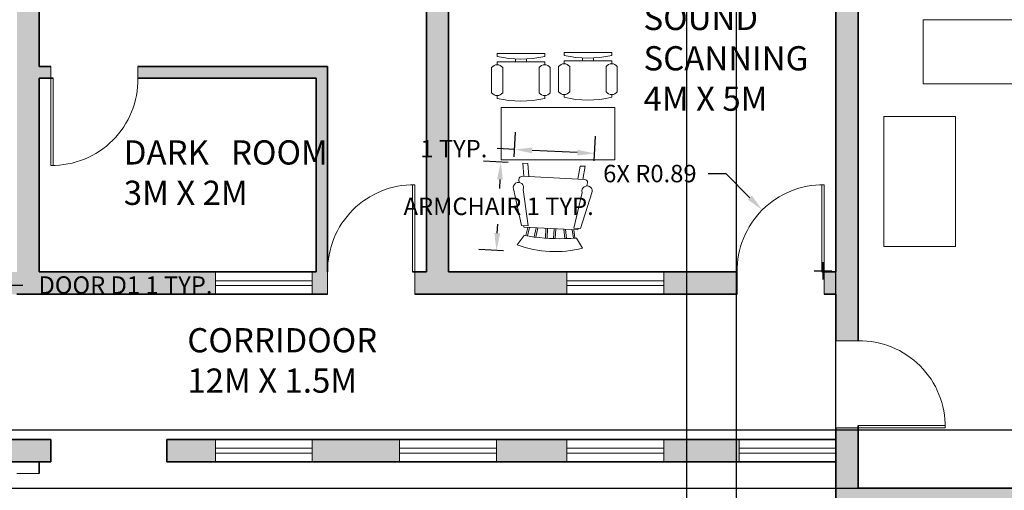
# Model space of a CAD drawing. Units: metres. Extents: x 4298.5 to 4325.2, y 2075 to 2095.8.
# Tile 32 of 35: x 4309.9 to 4320.1, y 2084.8 to 2089.6. Entities that reach past the tile are written whole.
import ezdxf

# ---------------------------------------------------------------- set-up
doc = ezdxf.new("R2010")
doc.units = ezdxf.units.M
for name, color, linetype, lineweight in [('A-ANNO-DIMS', 2, 'Continuous', 18), ('A-AREA-IDEN', 7, 'Continuous', 18), ('A-DOOR', 3, 'Continuous', 18), ('A-EQPM', 9, 'Continuous', 18), ('A-FURN', 15, 'Continuous', 18), ('A-GLAZ', 4, 'Continuous', 18), ('A-WALL', 7, 'Continuous', 35), ('A-WALL-PATT', 252, 'Continuous', 13)]:
    doc.layers.add(name, color=color, linetype=linetype, lineweight=lineweight)
doc.styles.get("Standard").update_dxf_attribs({"font": 'arial.ttf'})
doc.dimstyles.get("Standard").update_dxf_attribs({"dimtxt": 0.18, "dimasz": 0.18, "dimexe": 0.18, "dimexo": 0.0625, "dimgap": 0.09, "dimtad": 0, "dimtih": 1, "dimtoh": 1, "dimdec": 4, "dimzin": 0, "dimdsep": 46, "dimtxsty": 'Standard', "dimcen": 0.09, "dimadec": 0, "dimazin": 0, "dimtfac": 1, "dimtdec": 4, "dimtofl": 0, "dimtmove": 0, "dimatfit": 3, "dimfxl": 1, "dimtolj": 1, "dimtzin": 0, "dimarcsym": 0})

# ---------------------------------------------------------------- blocks, each defined once
blk = doc.blocks.new('Chair - Desk')
for p, q in [((-8.5, 0), (-8.5, -1)), ((-8.5, 0), (8.5, 0)), ((8.5, 0), (8.5, -1)), ((-8.5, -3), (-8.5, -4)), ((-8.5, -3), (8.5, -3)), ((-2, -3), (-2, -1.9355)), ((2, -1.9576), (2, -3)), ((8.5, -3), (8.5, -4)), ((-10.5, -5), (-10.5, -14)), ((-6.5, -14), (-6.5, -5)), ((6.5, -5), (6.5, -14)), ((10.5, -14), (10.5, -5)), ((-8.5, -15), (-8.5, -16)), ((8.5, -15), (8.5, -16))]:
    blk.add_line(p, q)
for centre, radius, start, end in [((0, 34.625), 36.625, 256.5803, 283.4197), ((-8.5, -6.5), 2.5, 36.8699, 143.1301), ((8.5, -6.5), 2.5, 36.8699, 143.1301), ((-8.5, -12.5), 2.5, 216.8699, 323.1301), ((8.5, -12.5), 2.5, 216.8699, 323.1301), ((0, 19.625), 36.625, 256.5803, 283.4197)]:
    blk.add_arc(centre, radius, start, end)
blk = doc.blocks.new('Chair - Rocking')
for p, q in [((-8, -4.5), (-10, -1.5)), ((8, -4.5), (10, -1.5)), ((-7.5, -4.5), (-7, -7)), ((-6.5, -7), (-7.02225, -4.43)), ((-4.5, -7), (-4.96674, -4.19951)), ((-4, -7), (-4.40532, -4.16272)), ((-1.5, -4.05012), (-1.5, -7)), ((-1, -7), (-1, -4.05012)), ((1, -7), (1, -4.04655)), ((1.5, -4.05012), (1.5, -7)), ((4, -7), (4.40187, -4.18694)), ((4.5, -7), (4.96761, -4.19437)), ((6.5, -7), (7, -4.4057)), ((7.5, -4.5), (7, -7)), ((-9, -7.5), (-12, -18.49999)), ((-7, -7.5), (-9, -7.5)), ((-9, -18.49999), (-7, -7.5)), ((-8.23428, -6.99939), (-8.3093, -7.47958)), ((-8.23041, -7), (8.23915, -7)), ((7, -7.5), (9, -7.5)), ((9, -18.49999), (7, -7.5)), ((8.31071, -7.48854), (8.23449, -7.00073)), ((9, -7.5), (12, -18.49999)), ((-10.36644, -20.64523), (-10.5, -21.49999)), ((10.5, -21.49999), (10.3575, -20.58798)), ((-9, -22.49999), (-9.5, -26.49999)), ((0, -22.49999), (-9.5, -22.49999)), ((-8, -26.49999), (-7.5, -22.49999)), ((0, -22.49999), (9.5, -22.49999)), ((8, -26.49999), (7.5, -22.49999)), ((9, -22.49999), (9.5, -26.49999)), ((-9.5, -26.49999), (-8, -26.49999)), ((9.5, -26.49999), (8, -26.49999))]:
    blk.add_line(p, q)
for centre, radius, start, end in [((0, -34.08333), 34.08333, 72.93847, 107.0615), ((0, -68.25004), 64.25, 93.92211, 97.15267), ((0, -68.25004), 64.25, 82.84733, 93.92211), ((-10.5, -18.99999), 1.58114, 161.5651, 18.43495), ((10.5, -18.99999), 1.58114, 161.5651, 18.43495), ((-9.5, -21.49999), 1, 180, 270), ((9.5, -21.49999), 1, 270, 0)]:
    blk.add_arc(centre, radius, start, end)
blk = doc.blocks.new('WIN-1000-GLASS')
for p, q in [((1, 0.05), (0, 0.05)), ((1, 0), (0, 0))]:
    blk.add_line(p, q)
blk = doc.blocks.new('DOOR-900-LEAF')
for p, q in [((0.9, 0.9), (0, 0.9)), ((0.9, 0.875), (0, 0.875))]:
    blk.add_line(p, q)
blk.add_arc((0.8875, 0.8875), 0.8876, 179.19307, 270.80693)
blk = doc.blocks.new('DESK-1175')
blk.add_lwpolyline([(0, 1.173), (0.538, 1.173), (0.538, 0), (0, 0)], close=True)
blk = doc.blocks.new('EQUIPMENT-1340')
blk.add_lwpolyline([(0, 1.342), (0.74, 1.342), (0.74, 0), (0, 0)], close=True)
blk = doc.blocks.new('*D29')
at = {"layer": 'A-ANNO-DIMS', "color": 0, "lineweight": -2, "transparency": 16777216}
for p, q in [((4308.867, 2086.956), (4308.867, 2086.703)), ((4309.047, 2086.883), (4309.591, 2086.883)), ((4309.771, 2086.956), (4309.771, 2086.703)), ((4309.771, 2086.883), (4309.951, 2086.883))]:
    blk.add_line(p, q, dxfattribs=at)
at = {"layer": 'A-ANNO-DIMS', "color": 0, "transparency": 16777216}
for points in [[(4309.047, 2086.913), (4309.047, 2086.853), (4308.867, 2086.883)], [(4309.591, 2086.913), (4309.591, 2086.853), (4309.771, 2086.883)]]:
    blk.add_solid(points, dxfattribs=at)
at = {"layer": 'Defpoints', "color": 0, "transparency": 16777216}
for p in [(4308.867, 2087.018), (4309.771, 2087.018), (4309.771, 2086.883)]:
    blk.add_point(p, dxfattribs=at)
at = {"layer": 'A-ANNO-DIMS', "color": 0, "transparency": 16777216, "insert": (4311.012, 2086.883), "char_height": 0.18, "attachment_point": 5}
blk.add_mtext('\\A1;DOOR D1 1 TYP.', dxfattribs=at)
blk = doc.blocks.new('*D35')
at = {"layer": 'A-ANNO-DIMS', "color": 0, "lineweight": -2, "transparency": 16777216}
for p, q in [((4314.964, 2088.149), (4314.71, 2088.161)), ((4314.88, 2087.972), (4314.876, 2087.879)), ((4314.853, 2087.42), (4314.857, 2087.513)), ((4314.918, 2087.236), (4314.664, 2087.249))]:
    blk.add_line(p, q, dxfattribs=at)
at = {"layer": 'A-ANNO-DIMS', "color": 0, "transparency": 16777216}
for points in [[(4314.85, 2087.974), (4314.91, 2087.971), (4314.889, 2088.152)], [(4314.823, 2087.421), (4314.883, 2087.418), (4314.844, 2087.24)]]:
    blk.add_solid(points, dxfattribs=at)
at = {"layer": 'Defpoints', "color": 0, "transparency": 16777216}
for p in [(4315.026, 2088.145), (4314.844, 2087.24), (4314.981, 2087.233)]:
    blk.add_point(p, dxfattribs=at)
at = {"layer": 'A-ANNO-DIMS', "color": 0, "transparency": 16777216, "insert": (4314.867, 2087.696), "char_height": 0.18, "attachment_point": 5}
blk.add_mtext('\\A1;ARMCHAIR 1 TYP.', dxfattribs=at)
blk = doc.blocks.new('*D36')
at = {"layer": 'A-ANNO-DIMS', "color": 0, "lineweight": -2, "transparency": 16777216}
for p, q in [((4315.029, 2088.208), (4315.042, 2088.462)), ((4315.855, 2088.167), (4315.868, 2088.421)), ((4315.033, 2088.282), (4314.853, 2088.291)), ((4315.679, 2088.25), (4315.213, 2088.273))]:
    blk.add_line(p, q, dxfattribs=at)
at = {"layer": 'A-ANNO-DIMS', "color": 0, "transparency": 16777216}
for points in [[(4315.214, 2088.303), (4315.211, 2088.243), (4315.033, 2088.282)], [(4315.681, 2088.28), (4315.678, 2088.22), (4315.859, 2088.241)]]:
    blk.add_solid(points, dxfattribs=at)
at = {"layer": 'Defpoints', "color": 0, "transparency": 16777216}
for p in [(4315.033, 2088.282), (4315.026, 2088.145), (4315.852, 2088.104)]:
    blk.add_point(p, dxfattribs=at)
at = {"layer": 'A-ANNO-DIMS', "color": 0, "transparency": 16777216, "insert": (4314.404, 2088.291), "char_height": 0.18, "attachment_point": 5}
blk.add_mtext('\\A1;1 TYP.', dxfattribs=at)
blk = doc.blocks.new('*D48')
at = {"layer": 'A-ANNO-DIMS', "color": 0, "lineweight": -2, "transparency": 16777216}
for p, q in [((4310.183, 2094.478), (4324.767, 2094.478)), ((4324.587, 2094.298), (4324.587, 2085.585)), ((4324.587, 2076.508), (4324.587, 2085.221)), ((4316.873, 2076.328), (4324.767, 2076.328))]:
    blk.add_line(p, q, dxfattribs=at)
at = {"layer": 'A-ANNO-DIMS', "color": 0, "transparency": 16777216}
for points in [[(4324.557, 2094.298), (4324.617, 2094.298), (4324.587, 2094.478)], [(4324.557, 2076.508), (4324.617, 2076.508), (4324.587, 2076.328)]]:
    blk.add_solid(points, dxfattribs=at)
at = {"layer": 'Defpoints', "color": 0, "transparency": 16777216}
for p in [(4310.121, 2094.478), (4316.811, 2076.328), (4324.587, 2076.328)]:
    blk.add_point(p, dxfattribs=at)
at = {"layer": 'A-ANNO-DIMS', "color": 0, "transparency": 16777216, "insert": (4324.587, 2085.403), "char_height": 0.18, "attachment_point": 5}
blk.add_mtext('\\A1;18.15', dxfattribs=at)
blk = doc.blocks.new('*D53')
at = {"layer": 'A-ANNO-DIMS', "color": 0, "lineweight": -2, "transparency": 16777216}
for p, q in [((4309.161, 2076.391), (4309.161, 2095.817)), ((4316.811, 2076.391), (4316.811, 2095.817)), ((4309.341, 2095.637), (4312.662, 2095.637)), ((4316.631, 2095.637), (4313.309, 2095.637))]:
    blk.add_line(p, q, dxfattribs=at)
at = {"layer": 'A-ANNO-DIMS', "color": 0, "transparency": 16777216}
for points in [[(4309.341, 2095.667), (4309.341, 2095.607), (4309.161, 2095.637)], [(4316.631, 2095.667), (4316.631, 2095.607), (4316.811, 2095.637)]]:
    blk.add_solid(points, dxfattribs=at)
at = {"layer": 'Defpoints', "color": 0, "transparency": 16777216}
for p in [(4316.811, 2095.637), (4309.161, 2076.328), (4316.811, 2076.328)]:
    blk.add_point(p, dxfattribs=at)
at = {"layer": 'A-ANNO-DIMS', "color": 0, "transparency": 16777216, "insert": (4312.986, 2095.637), "char_height": 0.18, "attachment_point": 5}
blk.add_mtext('\\A1;7.65', dxfattribs=at)
blk = doc.blocks.new('*D58')
at = {"layer": 'A-ANNO-DIMS', "color": 0, "lineweight": -2, "transparency": 16777216}
for p, q in [((4324.587, 2085.388), (4324.587, 2085.568)), ((4324.587, 2085.568), (4324.767, 2085.568)), ((4300.723, 2085.388), (4324.767, 2085.388)), ((4324.587, 2084.968), (4324.587, 2085.208)), ((4300.723, 2084.788), (4324.767, 2084.788))]:
    blk.add_line(p, q, dxfattribs=at)
at = {"layer": 'A-ANNO-DIMS', "color": 0, "transparency": 16777216}
for points in [[(4324.557, 2085.208), (4324.617, 2085.208), (4324.587, 2085.388)], [(4324.557, 2084.968), (4324.617, 2084.968), (4324.587, 2084.788)]]:
    blk.add_solid(points, dxfattribs=at)
at = {"layer": 'Defpoints', "color": 0, "transparency": 16777216}
for p in [(4300.661, 2085.388), (4324.587, 2085.388), (4300.661, 2084.788)]:
    blk.add_point(p, dxfattribs=at)
at = {"layer": 'A-ANNO-DIMS', "color": 0, "transparency": 16777216, "insert": (4325.021, 2085.568), "char_height": 0.18, "attachment_point": 5}
blk.add_mtext('\\A1;0.6', dxfattribs=at)
blk = doc.blocks.new('*D61')
at = {"layer": 'A-ANNO-DIMS', "color": 0, "lineweight": -2, "transparency": 16777216}
for p, q in [((4317.324045, 2083.575187), (4317.324045, 2095.816556)), ((4318.350577, 2084.620556), (4318.350577, 2095.816556)), ((4317.144045, 2095.636556), (4316.964045, 2095.636556)), ((4318.530577, 2095.636556), (4318.710577, 2095.636556))]:
    blk.add_line(p, q, dxfattribs=at)
at = {"layer": 'A-ANNO-DIMS', "color": 0, "transparency": 16777216}
for points in [[(4317.144045, 2095.666556), (4317.144045, 2095.606556), (4317.324045, 2095.636556)], [(4318.530577, 2095.666556), (4318.530577, 2095.606556), (4318.350577, 2095.636556)]]:
    blk.add_solid(points, dxfattribs=at)
at = {"layer": 'Defpoints', "color": 0, "transparency": 16777216}
for p in [(4318.350577, 2095.636556), (4318.350577, 2084.558056), (4317.324045, 2083.512687)]:
    blk.add_point(p, dxfattribs=at)
at = {"layer": 'A-ANNO-DIMS', "color": 0, "transparency": 16777216, "insert": (4317.837311, 2095.636556), "char_height": 0.18, "attachment_point": 5}
blk.add_mtext('\\A1;1.03', dxfattribs=at)
blk = doc.blocks.new('*D80')
at = {"layer": 'A-ANNO-DIMS', "color": 0, "lineweight": -2, "transparency": 16777216}
for p, q in [((4317.033, 2088.034), (4317.213, 2088.034)), ((4317.213, 2088.034), (4317.463, 2087.785)), ((4318.218, 2086.941), (4318.218, 2087.121)), ((4318.128, 2087.031), (4318.308, 2087.031))]:
    blk.add_line(p, q, dxfattribs=at)
at = {"layer": 'A-ANNO-DIMS', "color": 0, "transparency": 16777216}
blk.add_solid([(4317.484, 2087.806), (4317.442, 2087.764), (4317.59, 2087.658)], dxfattribs=at)
at = {"layer": 'Defpoints', "color": 0, "transparency": 16777216}
for p in [(4317.59, 2087.658), (4318.218, 2087.031)]:
    blk.add_point(p, dxfattribs=at)
at = {"layer": 'A-ANNO-DIMS', "color": 0, "transparency": 16777216, "insert": (4316.429, 2088.034), "char_height": 0.18, "attachment_point": 5}
blk.add_mtext('\\A1;6X R0.89', dxfattribs=at)

msp = doc.modelspace()

# ---------------------------------------------------------------- hatches: boundary and pattern name
at = {"layer": 'A-WALL-PATT'}
h = msp.add_hatch(color=256, dxfattribs=at)
h.dxf.hatch_style = 1
h.paths.add_polyline_path([(4308.7606, 2094.4781), (4308.1606, 2094.4781), (4307.4606, 2094.4781), (4307.4606, 2094.2481), (4308.2706, 2094.2481), (4308.2706, 2094.1281), (4308.3906, 2094.1281), (4308.3906, 2094.2481), (4308.7606, 2094.2481)])
h.paths.add_polyline_path([(4310.1206, 2094.4781), (4309.5206, 2094.4781), (4309.5206, 2094.2481), (4309.8906, 2094.2481), (4309.8906, 2092.2481), (4308.3906, 2092.2481), (4308.3906, 2093.4281), (4308.2706, 2093.4281), (4308.2706, 2092.0181), (4309.8906, 2092.0181), (4309.8906, 2087.0181), (4309.7706, 2087.0181), (4309.7706, 2086.7881), (4309.8906, 2086.7881), (4311.9406, 2086.7881), (4311.9406, 2087.0181), (4310.1206, 2087.0181), (4310.1206, 2089.0181), (4310.2406, 2089.0181), (4310.2406, 2089.1381), (4310.1206, 2089.1381), (4310.1206, 2092.0181), (4310.3078, 2092.0181), (4310.3078, 2092.2481), (4310.1206, 2092.2481)])
h.paths.add_polyline_path([(4311.7406, 2092.2481), (4311.0678, 2092.2481), (4311.0678, 2092.0181), (4311.7406, 2092.0181)], flags=17)
h.paths.add_polyline_path([(4313.1733, 2092.2481), (4312.5006, 2092.2481), (4312.5006, 2092.0181), (4313.1733, 2092.0181)])
h.paths.add_polyline_path([(4314.5378, 2092.2481), (4314.1206, 2092.2481), (4313.9333, 2092.2481), (4313.9333, 2092.0181), (4314.1206, 2092.0181), (4314.1206, 2087.0181), (4314.0006, 2087.0181), (4314.0006, 2086.7881), (4314.1206, 2086.7881), (4315.5718, 2086.7881), (4315.5718, 2087.0181), (4314.3506, 2087.0181), (4314.3506, 2092.0181), (4314.5378, 2092.0181)])
h.paths.add_polyline_path([(4315.9706, 2092.2481), (4315.2978, 2092.2481), (4315.2978, 2092.0181), (4315.9706, 2092.0181)])
h.paths.add_polyline_path([(4317.4033, 2092.2481), (4316.7306, 2092.2481), (4316.7306, 2092.0181), (4317.4033, 2092.0181)])
h.paths.add_polyline_path([(4318.9506, 2092.2481), (4318.3506, 2092.2481), (4318.1633, 2092.2481), (4318.1633, 2092.0181), (4318.3506, 2092.0181), (4318.3506, 2091.8981), (4318.5806, 2091.8981), (4318.5806, 2092.0181), (4318.9506, 2092.0181)])
h.paths.add_polyline_path([(4321.0106, 2092.2481), (4319.7106, 2092.2481), (4319.7106, 2092.0181), (4320.0806, 2092.0181), (4320.0806, 2090.0181), (4318.5806, 2090.0181), (4318.5806, 2091.1981), (4318.3506, 2091.1981), (4318.3506, 2090.0181), (4318.3506, 2087.0181), (4318.2306, 2087.0181), (4318.2306, 2086.7881), (4318.3506, 2086.7881), (4318.3506, 2086.3081), (4318.5806, 2086.3081), (4318.5806, 2089.7881), (4321.7806, 2089.7881), (4321.7806, 2090.0181), (4320.2006, 2090.0181), (4320.2006, 2092.0181), (4321.0106, 2092.0181)])
h.paths.add_polyline_path([(4322.8106, 2092.2481), (4321.7706, 2092.2481), (4321.7706, 2092.0181), (4322.5806, 2092.0181), (4322.5806, 2091.2831), (4322.8106, 2091.2831)])
h.paths.add_polyline_path([(4322.8106, 2090.5231), (4322.5806, 2090.5231), (4322.5806, 2089.7881), (4322.5806, 2089.5254), (4322.8106, 2089.5254), (4322.8106, 2090.0181)])
h.paths.add_polyline_path([(4322.8106, 2088.7654), (4322.5806, 2088.7654), (4322.5806, 2087.6681), (4322.8106, 2087.6681)])
h.paths.add_polyline_path([(4322.8106, 2086.9081), (4322.5806, 2086.9081), (4322.5806, 2085.8107), (4322.8106, 2085.8107)])
h.paths.add_polyline_path([(4322.8106, 2085.0507), (4322.5806, 2085.0507), (4322.5806, 2084.7881), (4318.5806, 2084.7881), (4318.5806, 2085.0581), (4318.5806, 2085.4081), (4318.3506, 2085.4081), (4318.3506, 2084.5581), (4318.3506, 2080.8581), (4318.4706, 2080.8581), (4318.4706, 2082.3281), (4319.2606, 2082.3281), (4319.2606, 2082.5581), (4318.5806, 2082.5581), (4318.5806, 2084.5581), (4320.0806, 2084.5581), (4320.0806, 2083.9381), (4320.3106, 2083.9381), (4320.3106, 2084.5581), (4322.8106, 2084.5581)])
h.paths.add_polyline_path([(4320.3106, 2083.1781), (4320.0806, 2083.1781), (4320.0806, 2082.5581), (4319.9606, 2082.5581), (4319.9606, 2082.3281), (4320.0806, 2082.3281), (4320.0806, 2081.5731), (4320.3106, 2081.5731)], flags=17)
h.paths.add_polyline_path([(4320.3106, 2080.8131), (4320.0806, 2080.8131), (4320.0806, 2080.0581), (4318.4286, 2080.0581), (4318.4286, 2079.8281), (4320.3106, 2079.8281)])
h.paths.add_polyline_path([(4317.3506, 2085.2881), (4316.5718, 2085.2881), (4316.5718, 2085.0581), (4317.3506, 2085.0581)])
h.paths.add_polyline_path([(4315.5718, 2085.2881), (4314.8434, 2085.2881), (4314.8434, 2085.0581), (4315.5718, 2085.0581)])
h.paths.add_polyline_path([(4313.8434, 2085.2881), (4312.9406, 2085.2881), (4312.9406, 2085.0581), (4313.8434, 2085.0581)])
h.paths.add_polyline_path([(4311.9406, 2085.2881), (4311.4406, 2085.2881), (4311.4406, 2085.0581), (4311.9406, 2085.0581)])
h.paths.add_polyline_path([(4317.3306, 2087.0181), (4316.5718, 2087.0181), (4316.5718, 2086.7881), (4317.3306, 2086.7881)])
h.paths.add_polyline_path([(4313.1006, 2089.1381), (4311.1406, 2089.1381), (4311.1406, 2089.0181), (4312.9806, 2089.0181), (4312.9806, 2087.0181), (4312.9406, 2087.0181), (4312.9406, 2086.7881), (4313.1006, 2086.7881), (4313.1006, 2087.0181)])
h.paths.add_polyline_path([(4307.5515, 2087.0181), (4305.8906, 2087.0181), (4305.8906, 2092.2481), (4305.8906, 2094.2481), (4306.7006, 2094.2481), (4306.7006, 2094.4781), (4305.6606, 2094.4781), (4305.6606, 2092.2481), (4305.2906, 2092.2481), (4305.2906, 2092.0181), (4305.6606, 2092.0181), (4305.6606, 2090.0181), (4304.1606, 2090.0181), (4304.1606, 2091.1981), (4304.0406, 2091.1981), (4304.0406, 2089.9081), (4301.5606, 2089.9081), (4301.5606, 2089.7881), (4304.0406, 2089.7881), (4305.6606, 2089.7881), (4305.6606, 2086.6381), (4305.8906, 2086.6381), (4305.8906, 2086.7881), (4307.5515, 2086.7881)])
h.paths.add_polyline_path([(4307.5515, 2085.2881), (4305.8906, 2085.2881), (4305.8906, 2085.4381), (4305.6606, 2085.4381), (4305.6606, 2084.7881), (4305.2906, 2084.7881), (4305.2906, 2084.5581), (4305.6606, 2084.5581), (4305.6606, 2084.02), (4305.8906, 2084.02), (4305.8906, 2084.5581), (4305.8906, 2085.0581), (4307.5515, 2085.0581)])
h.paths.add_polyline_path([(4310.2406, 2085.2881), (4308.5515, 2085.2881), (4308.5515, 2085.0581), (4310.2406, 2085.0581)])
h.paths.add_polyline_path([(4317.4286, 2080.0581), (4316.5718, 2080.0581), (4316.5718, 2079.8281), (4317.4286, 2079.8281)])
h.paths.add_polyline_path([(4315.5718, 2080.0581), (4314.8434, 2080.0581), (4314.8434, 2079.8281), (4315.5718, 2079.8281)])
h.paths.add_polyline_path([(4313.8434, 2080.0581), (4312.9406, 2080.0581), (4312.9406, 2079.8281), (4313.8434, 2079.8281)])
h.paths.add_polyline_path([(4311.9406, 2080.0581), (4311.4406, 2080.0581), (4311.4406, 2079.8281), (4311.9406, 2079.8281)])
h.paths.add_polyline_path([(4310.2406, 2080.0581), (4310.1206, 2080.0581), (4310.1206, 2084.0381), (4309.8906, 2084.0381), (4309.8906, 2080.0581), (4309.1606, 2080.0581), (4309.1606, 2079.8281), (4310.2406, 2079.8281)])
h.paths.add_polyline_path([(4308.1606, 2080.0581), (4307.5106, 2080.0581), (4307.5106, 2080.1781), (4307.3906, 2080.1781), (4307.3906, 2080.0581), (4305.8906, 2080.0581), (4305.8906, 2080.567), (4305.6606, 2080.567), (4305.6606, 2079.8281), (4308.1606, 2079.8281)])
h.paths.add_polyline_path([(4307.5106, 2081.9381), (4309.0906, 2081.9381), (4309.0906, 2082.0581), (4305.8906, 2082.0581), (4305.8906, 2083.26), (4305.6606, 2083.26), (4305.6606, 2081.327), (4305.8906, 2081.327), (4305.8906, 2081.9381), (4307.3906, 2081.9381), (4307.3906, 2080.8781), (4307.5106, 2080.8781)])
h.paths.add_polyline_path([(4304.5306, 2084.7881), (4302.7306, 2084.7881), (4302.7306, 2084.5581), (4304.5306, 2084.5581)])
h.paths.add_polyline_path([(4301.9706, 2084.7881), (4300.6606, 2084.7881), (4300.6606, 2085.0249), (4300.4306, 2085.0249), (4300.4306, 2084.5581), (4301.9706, 2084.5581)])
h.paths.add_polyline_path([(4300.6606, 2086.8843), (4300.4306, 2086.8843), (4300.4306, 2085.7849), (4300.6606, 2085.7849)])
h.paths.add_polyline_path([(4300.6606, 2089.1618), (4300.4306, 2089.1618), (4300.4306, 2087.6443), (4300.6606, 2087.6443)])
h.paths.add_polyline_path([(4300.6606, 2091.0212), (4300.4306, 2091.0212), (4300.4306, 2089.9218), (4300.6606, 2089.9218)])
h.paths.add_polyline_path([(4300.6606, 2092.0181), (4301.9706, 2092.0181), (4301.9706, 2092.2481), (4300.4306, 2092.2481), (4300.4306, 2091.7812), (4300.6606, 2091.7812)])
h.paths.add_polyline_path([(4304.5306, 2092.2481), (4302.7306, 2092.2481), (4302.7306, 2092.0181), (4304.0406, 2092.0181), (4304.0406, 2091.8981), (4304.1606, 2091.8981), (4304.1606, 2092.0181), (4304.5306, 2092.0181)], flags=17)

# ---------------------------------------------------------------- linework, layer by layer
at = {"layer": 'A-DOOR'}
for p, q in [((4310.2406, 2089.0181), (4310.2406, 2089.1381)), ((4311.1406, 2089.0181), (4311.1406, 2089.1381)), ((4313.1006, 2087.0181), (4313.1006, 2086.7881)), ((4314.0006, 2087.0181), (4314.0006, 2086.7881)), ((4317.3306, 2087.0181), (4317.3306, 2086.7881)), ((4318.2306, 2086.7881), (4318.2306, 2087.0181)), ((4318.5806, 2086.3081), (4318.3506, 2086.3081)), ((4318.3506, 2085.4081), (4318.5806, 2085.4081)), ((4309.8906, 2084.9381), (4310.1206, 2084.9381))]:
    msp.add_line(p, q, dxfattribs=at)
at = {"layer": 'A-EQPM'}
msp.add_lwpolyline([(4319.2513, 2089.6206), (4320.7499, 2089.6206), (4320.7499, 2088.9592), (4319.2513, 2088.9592)], close=True, dxfattribs=at)
at = {"layer": 'A-GLAZ'}
for p, q in [((4311.9406, 2086.7881), (4311.9406, 2087.0181)), ((4312.9406, 2087.0181), (4312.9406, 2086.7881)), ((4315.5718, 2087.0181), (4315.5718, 2086.7881)), ((4316.5718, 2087.0181), (4316.5718, 2086.7881)), ((4311.9406, 2085.2881), (4311.9406, 2085.0581)), ((4312.9406, 2085.0581), (4312.9406, 2085.2881)), ((4313.8434, 2085.0581), (4313.8434, 2085.2881)), ((4314.8434, 2085.0581), (4314.8434, 2085.2881)), ((4315.5718, 2085.0581), (4315.5718, 2085.2881)), ((4316.5718, 2085.0581), (4316.5718, 2085.2881)), ((4317.3506, 2085.0581), (4317.3506, 2085.2881)), ((4318.3506, 2085.0581), (4318.3506, 2085.2881))]:
    msp.add_line(p, q, dxfattribs=at)
at = {"layer": 'A-WALL'}
for p, q in [((4310.1206, 2092.0181), (4310.1206, 2089.1381)), ((4314.1206, 2092.0181), (4314.1206, 2087.0181)), ((4314.3506, 2092.0181), (4314.3506, 2087.0181)), ((4318.3506, 2087.0181), (4318.3506, 2090.0181)), ((4318.5806, 2086.3081), (4318.5806, 2089.7881)), ((4310.1206, 2089.1381), (4310.2406, 2089.1381)), ((4311.1406, 2089.1381), (4313.1006, 2089.1381)), ((4313.1006, 2087.0181), (4313.1006, 2089.1381)), ((4310.1206, 2089.0181), (4310.2656, 2089.0181)), ((4310.1206, 2089.0181), (4310.1206, 2087.0181)), ((4311.1406, 2089.0181), (4312.9806, 2089.0181)), ((4312.9806, 2087.0181), (4312.9806, 2089.0181)), ((4310.1206, 2087.0181), (4312.9806, 2087.0181)), ((4313.9756, 2087.0181), (4314.1206, 2087.0181)), ((4314.3506, 2087.0181), (4317.3306, 2087.0181)), ((4318.2056, 2087.0181), (4318.3506, 2087.0181)), ((4309.8906, 2086.7881), (4313.1006, 2086.7881)), ((4314.0006, 2086.7881), (4314.1206, 2086.7881)), ((4314.1206, 2086.7881), (4317.3306, 2086.7881)), ((4318.2306, 2086.7881), (4318.3506, 2086.7881)), ((4318.3506, 2086.3081), (4318.3506, 2086.7881)), ((4318.3506, 2084.5581), (4318.3506, 2085.4081)), ((4318.5806, 2084.7881), (4318.5806, 2085.4331)), ((4305.8906, 2085.2881), (4310.2406, 2085.2881)), ((4310.2406, 2085.2881), (4310.2406, 2085.0581)), ((4311.4406, 2085.2881), (4311.4406, 2085.0581)), ((4311.4406, 2085.2881), (4318.3506, 2085.2881)), ((4305.8906, 2085.0581), (4310.2406, 2085.0581)), ((4310.1206, 2085.0581), (4310.1206, 2084.9381)), ((4311.4406, 2085.0581), (4318.3506, 2085.0581)), ((4318.3506, 2085.0581), (4318.3506, 2080.8581)), ((4318.5806, 2085.0581), (4318.5806, 2084.7881)), ((4322.5806, 2084.7881), (4318.5806, 2084.7881))]:
    msp.add_line(p, q, dxfattribs=at)

# ---------------------------------------------------------------- block references
at = {"layer": 'A-DOOR'}
for p, rotation in [((4311.1406, 2088.1181), 89.99999999999955), ((4313.1006, 2087.9181), 270), ((4317.3306, 2087.9181), 270), ((4319.4806, 2086.3081), 180)]:
    msp.add_blockref('DOOR-900-LEAF', p, dxfattribs=dict(at, rotation=rotation))
at = {"layer": 'A-EQPM'}
msp.add_blockref('EQUIPMENT-1340', (4318.8476, 2087.2817), dxfattribs=at)
at = {"layer": 'A-FURN', "xscale": 0.0288995186862949, "yscale": 0.0288995186862949, "zscale": 0.0288995186862949}
for p in [(4315.0972, 2089.2726), (4315.7895, 2089.2833)]:
    msp.add_blockref('Chair - Desk', p, dxfattribs=at)
at = {"layer": 'A-FURN', "rotation": 89.99999999992224}
msp.add_blockref('DESK-1175', (4316.0657, 2088.1771), dxfattribs=at)
at = {"layer": 'A-FURN', "xscale": 0.0338365474760119, "yscale": 0.0338365474760119, "zscale": 0.0338365474760119, "rotation": 177.1375936308194}
msp.add_blockref('Chair - Rocking', (4315.3944, 2087.2292), dxfattribs=at)
at = {"layer": 'A-GLAZ'}
for p in [(4311.9406, 2086.8781), (4315.5718, 2086.8781)]:
    msp.add_blockref('WIN-1000-GLASS', p, dxfattribs=at)
at = {"layer": 'A-GLAZ', "rotation": 180}
for p in [(4312.9406, 2085.1981), (4314.8434, 2085.1981), (4316.5718, 2085.1981), (4318.3506, 2085.1981)]:
    msp.add_blockref('WIN-1000-GLASS', p, dxfattribs=at)

# ---------------------------------------------------------------- texts
at = {"layer": 'A-AREA-IDEN', "char_height": 0.25, "attachment_point": 1}
for s, width, heights, insert in [('ULTRA SOUND SCANNING\\P4M X 5M', 2.22034, [0], (4316.3635, 2090.1823)), ('DARK   ROOM\\P3M X 2M', 2.22034, [0], (4310.9944, 2088.3771)), ('CORRIDOOR\\P12M X 1.5M', 6.564266, [0.6764], (4311.6511, 2086.4385))]:
    msp.add_mtext_dynamic_manual_height_columns(s, width=width, gutter_width=12.5, heights=heights, dxfattribs=dict(at, insert=insert))

# ---------------------------------------------------------------- dimensions: what is measured, and where the dimension line sits
at = {"layer": 'A-ANNO-DIMS'}
for base, p1, p2, picture, middle in [((4316.8106, 2095.6366), (4309.1606, 2076.3281), (4316.8106, 2076.3281), '*D53', (4312.9856, 2095.6366)), ((4318.3506, 2095.6366), (4317.324, 2083.5127), (4318.3506, 2084.5581), '*D61', (4317.8373, 2095.6366))]:
    dim = msp.add_linear_dim(base=base, p1=p1, p2=p2, dimstyle='Standard', override={"dimdec": 2, "dimlfac": 1, "dimrnd": 0, "dimzin": 0, "dimdsep": 46, "dimlunit": 2}, dxfattribs=at)
    dim.commit()
    dim.dimension.update_dxf_attribs({"geometry": picture, "text_midpoint": middle})
for base, p1, p2, override, picture, middle in [((4324.5871, 2076.3281), (4310.1206, 2094.4781), (4316.8106, 2076.3281), {"dimdec": 2, "dimlfac": 1, "dimrnd": 0, "dimzin": 0, "dimdsep": 46, "dimlunit": 2}, '*D48', (4324.5871, 2085.4031)), ((4324.5871, 2085.3881), (4300.6606, 2084.7881), (4300.6606, 2085.3881), {"dimdec": 1, "dimlfac": 1, "dimrnd": 0, "dimzin": 0, "dimdsep": 46, "dimlunit": 2}, '*D58', (4325.0209, 2085.5681))]:
    dim = msp.add_linear_dim(base=base, p1=p1, p2=p2, angle=90, dimstyle='Standard', override=override, dxfattribs=at)
    dim.commit()
    dim.dimension.update_dxf_attribs({"geometry": picture, "text_midpoint": middle})
for base, p1, p2, angle, text, picture, middle in [((4315.0331, 2088.2823), (4315.8521, 2088.1041), (4315.0263, 2088.1454), 177.13759, '<> TYP.', '*D36', (4314.4037, 2088.2913)), ((4314.8438, 2087.2398), (4315.0263, 2088.1454), (4314.9807, 2087.233), 267.13759, 'ARMCHAIR <> TYP.', '*D35', (4314.8666, 2087.6961)), ((4309.7706, 2086.8825), (4308.8672, 2087.0181), (4309.7706, 2087.0181), 0, 'DOOR D1 <> TYP.', '*D29', (4311.012, 2086.8825))]:
    dim = msp.add_linear_dim(base=base, p1=p1, p2=p2, angle=angle, text=text, dimstyle='Standard', override={"dimdec": 0, "dimlfac": 1, "dimrnd": 0, "dimzin": 0, "dimdsep": 46, "dimlunit": 2}, dxfattribs=at)
    dim.commit()
    dim.dimension.update_dxf_attribs({"geometry": picture, "text_midpoint": middle})
dim = msp.add_radius_dim(center=(4318.2181, 2087.0306), mpoint=(4317.5901, 2087.6579), text='6X <>', dimstyle='Standard', override={"dimdec": 2, "dimlfac": 1, "dimrnd": 0, "dimzin": 0, "dimdsep": 46, "dimlunit": 2}, dxfattribs=at)
dim.commit()
dim.dimension.update_dxf_attribs({"geometry": '*D80', "text_midpoint": (4316.4294, 2088.0342), "dimtype": 164})

doc.saveas('drawing.dxf')
